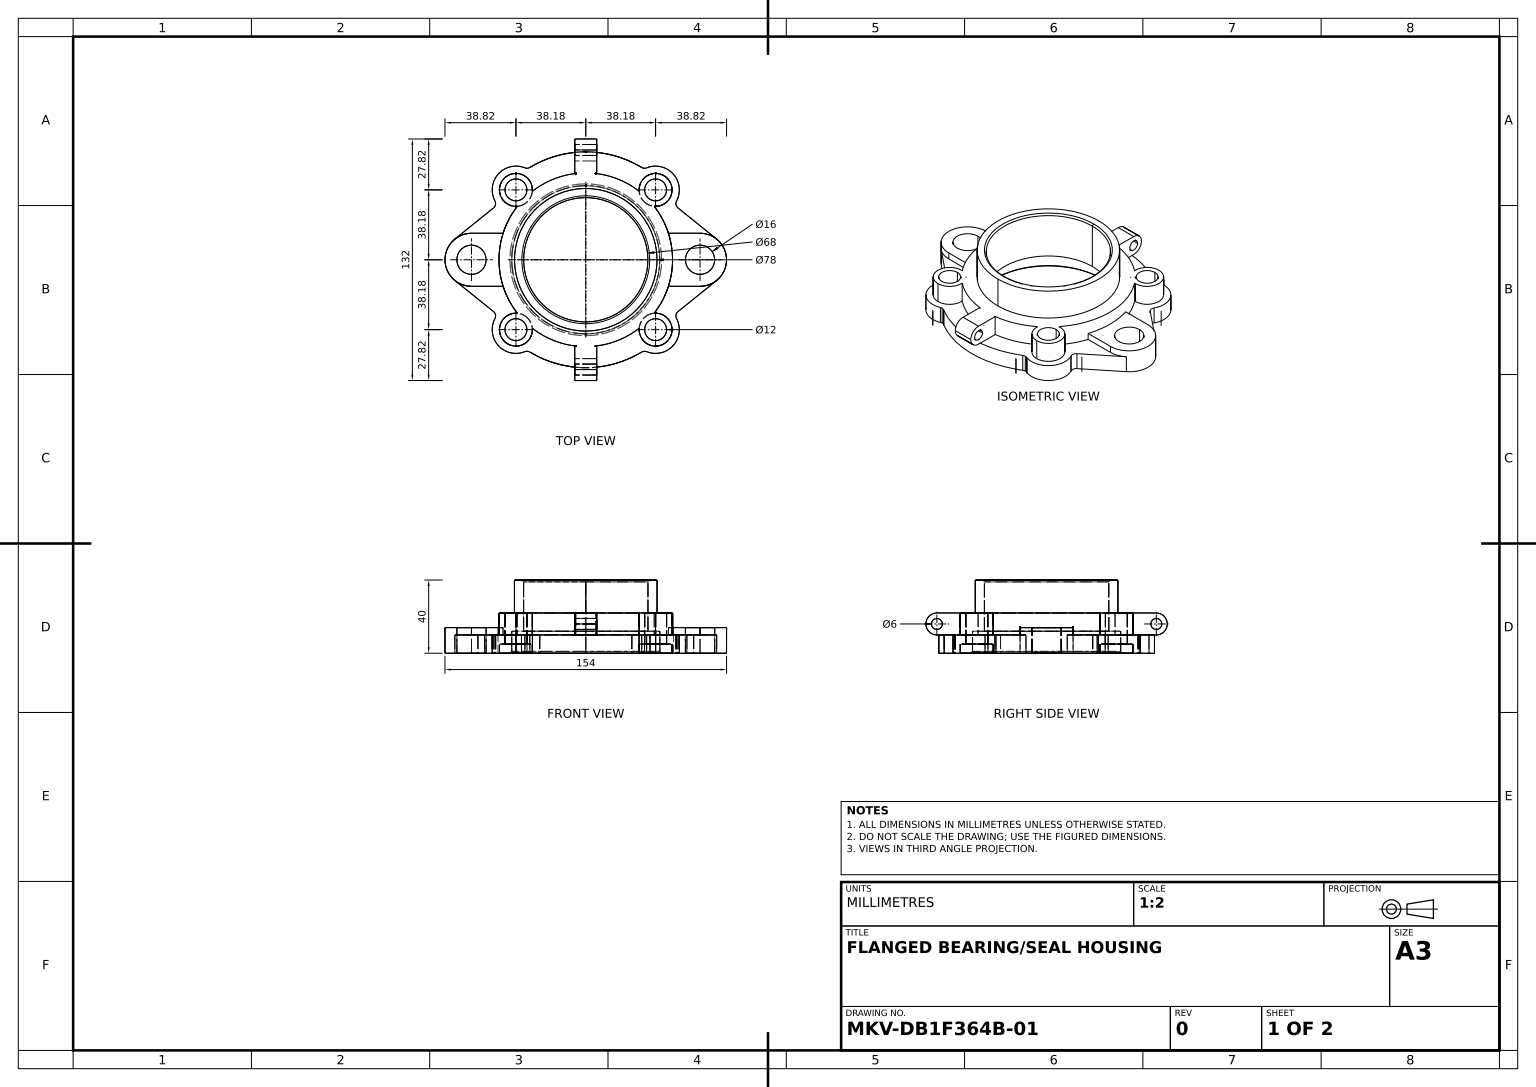
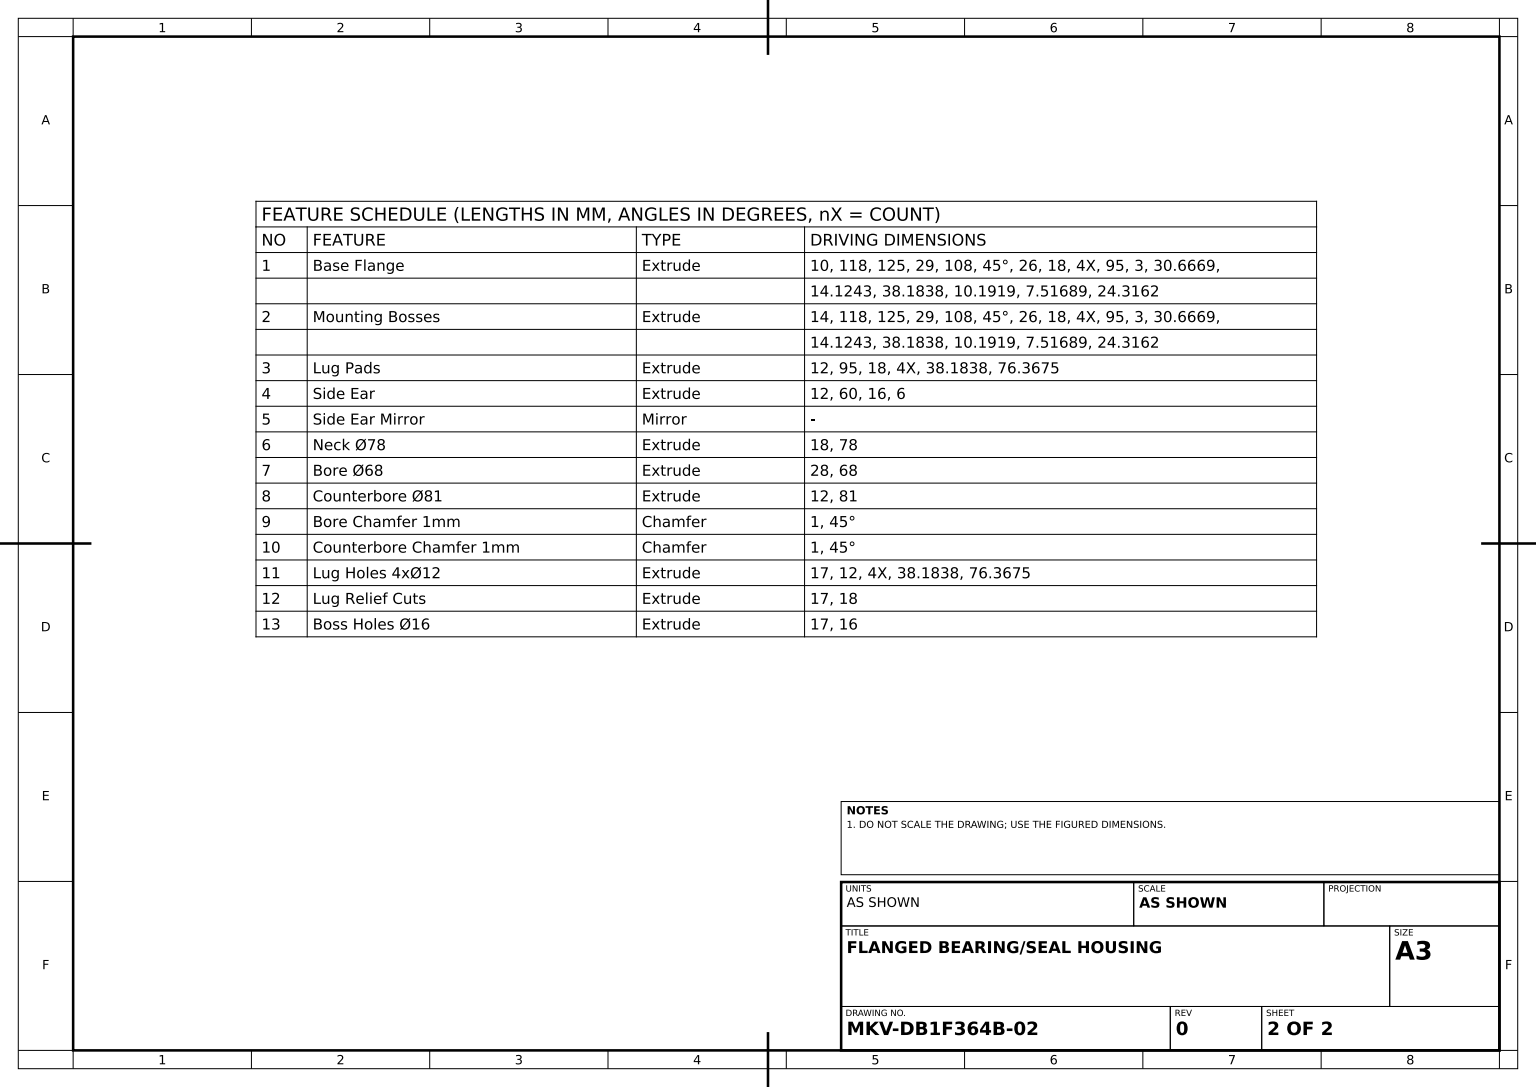
from build123d import *

# Parameters (mm, degrees)
BASE_FLANGE_DEPTH            = 10
MOUNTING_BOSSES_DEPTH        = 14
LUG_PADS_DEPTH               = 12
SIDE_EAR_SKETCH_R            = 3
SIDE_EAR_DEPTH               = 6
NECK_SKETCH_78_R             = 39
NECK_78_DEPTH                = 18
BORE_SKETCH_68_R             = 34
BORE_68_DEPTH                = 28
COUNTERBORE_SKETCH_81_R      = 40.5
COUNTERBORE_81_DEPTH         = 12
BORE_CHAMFER_1MM_SIZE        = 1
COUNTERBORE_CHAMFER_1MM_SIZE = 1
LUG_HOLES_SKETCH_R           = 6
LUG_HOLES_4X_12_DEPTH        = 17
LUG_START                    = -17
LUG_RELIEF_SKETCH_R          = 9
LUG_RELIEF_CUTS_DEPTH        = 17
BOSS_HOLES_SKETCH_R          = 8
BOSS_HOLES_16_DEPTH          = 17


with BuildPart() as part:
    # Base Flange Sketch → Base Flange (new body)
    with BuildSketch(Plane(origin=(0, 0, 0), x_dir=(1, 0, 0), z_dir=(0, 1, 0))):
        with BuildLine():
            Line((-45.232731512, -14.5), (-62.5, -14.5))
            ThreePointArc((-62.5, -14.5), (-67.319751251, -13.675525507), (-71.591397402, -11.295861777))
            Line((-71.591397402, -11.295861777), (-50.427104316, -28.329798892))
            ThreePointArc((-50.427104316, -28.329798892), (-49.36909282, -30.064930059), (-49.659773669, -32.076291075))
            ThreePointArc((-49.659773669, -32.076291075), (-47.837591407, -46.890295835), (-33.289777567, -50.227390033))
            ThreePointArc((-33.289777567, -50.227390033), (-31.921585171, -50.016208018), (-30.604247405, -50.44184811))
            ThreePointArc((-30.604247405, -50.44184811), (0, -59), (30.604247405, -50.44184811))
            ThreePointArc((30.604247405, -50.44184811), (31.921585171, -50.016208018), (33.289777567, -50.227390033))
            ThreePointArc((33.289777567, -50.227390033), (47.837591407, -46.890295835), (49.659773669, -32.076291075))
            ThreePointArc((49.659773669, -32.076291075), (49.36909282, -30.064930059), (50.427104316, -28.329798892))
            Line((50.427104316, -28.329798892), (71.591397402, -11.295861777))
            ThreePointArc((71.591397402, -11.295861777), (67.319751251, -13.675525507), (62.5, -14.5))
            Line((62.5, -14.5), (45.232731512, -14.5))
            ThreePointArc((45.232731512, -14.5), (43.022471721, -20.132484374), (40.114125183, -25.438297128))
            ThreePointArc((40.114125183, -25.438297128), (39.792711515, -27.966518872), (41.531678205, -29.829636361))
            ThreePointArc((41.531678205, -29.829636361), (44.547727215, -44.547727215), (29.829636361, -41.531678205))
            ThreePointArc((29.829636361, -41.531678205), (27.966518872, -39.792711515), (25.438297128, -40.114125183))
            ThreePointArc((25.438297128, -40.114125183), (0, -47.5), (-25.438297128, -40.114125183))
            ThreePointArc((-25.438297128, -40.114125183), (-27.966518872, -39.792711515), (-29.829636361, -41.531678205))
            ThreePointArc((-29.829636361, -41.531678205), (-44.547727215, -44.547727215), (-41.531678205, -29.829636361))
            ThreePointArc((-41.531678205, -29.829636361), (-39.792711515, -27.966518872), (-40.114125183, -25.438297128))
            ThreePointArc((-40.114125183, -25.438297128), (-43.022471721, -20.132484374), (-45.232731512, -14.5))
        make_face()
        with BuildLine():
            Line((-62.5, 14.5), (-45.232731512, 14.5))
            ThreePointArc((-45.232731512, 14.5), (-43.022471721, 20.132484374), (-40.114125183, 25.438297128))
            ThreePointArc((-40.114125183, 25.438297128), (-39.792711515, 27.966518872), (-41.531678205, 29.829636361))
            ThreePointArc((-41.531678205, 29.829636361), (-44.547727215, 44.547727215), (-29.829636361, 41.531678205))
            ThreePointArc((-29.829636361, 41.531678205), (-27.966518872, 39.792711515), (-25.438297128, 40.114125183))
            ThreePointArc((-25.438297128, 40.114125183), (0, 47.5), (25.438297128, 40.114125183))
            ThreePointArc((25.438297128, 40.114125183), (27.966518872, 39.792711515), (29.829636361, 41.531678205))
            ThreePointArc((29.829636361, 41.531678205), (44.547727215, 44.547727215), (41.531678205, 29.829636361))
            ThreePointArc((41.531678205, 29.829636361), (39.792711515, 27.966518872), (40.114125183, 25.438297128))
            ThreePointArc((40.114125183, 25.438297128), (43.022471721, 20.132484374), (45.232731512, 14.5))
            Line((45.232731512, 14.5), (62.5, 14.5))
            ThreePointArc((62.5, 14.5), (67.319751251, 13.675525507), (71.591397402, 11.295861777))
            Line((71.591397402, 11.295861777), (50.427104316, 28.329798892))
            ThreePointArc((50.427104316, 28.329798892), (49.36909282, 30.064930059), (49.659773669, 32.076291075))
            ThreePointArc((49.659773669, 32.076291075), (47.837591407, 46.890295835), (33.289777567, 50.227390033))
            ThreePointArc((33.289777567, 50.227390033), (31.921585171, 50.016208018), (30.604247405, 50.44184811))
            ThreePointArc((30.604247405, 50.44184811), (0, 59), (-30.604247405, 50.44184811))
            ThreePointArc((-30.604247405, 50.44184811), (-31.921585171, 50.016208018), (-33.289777567, 50.227390033))
            ThreePointArc((-33.289777567, 50.227390033), (-47.837591407, 46.890295835), (-49.659773669, 32.076291075))
            ThreePointArc((-49.659773669, 32.076291075), (-49.36909282, 30.064930059), (-50.427104316, 28.329798892))
            Line((-50.427104316, 28.329798892), (-71.591397402, 11.295861777))
            ThreePointArc((-71.591397402, 11.295861777), (-67.319751251, 13.675525507), (-62.5, 14.5))
        make_face()
        with BuildLine():
            ThreePointArc((-25.438297128, -40.114125183), (-27.966518872, -39.792711515), (-29.829636361, -41.531678205))
            ThreePointArc((-29.829636361, -41.531678205), (-44.547727215, -44.547727215), (-41.531678205, -29.829636361))
            ThreePointArc((-41.531678205, -29.829636361), (-39.792711515, -27.966518872), (-40.114125183, -25.438297128))
            ThreePointArc((-40.114125183, -25.438297128), (-47.5, 0), (-40.114125183, 25.438297128))
            ThreePointArc((-40.114125183, 25.438297128), (-39.792711515, 27.966518872), (-41.531678205, 29.829636361))
            ThreePointArc((-41.531678205, 29.829636361), (-44.547727215, 44.547727215), (-29.829636361, 41.531678205))
            ThreePointArc((-29.829636361, 41.531678205), (-27.966518872, 39.792711515), (-25.438297128, 40.114125183))
            ThreePointArc((-25.438297128, 40.114125183), (0, 47.5), (25.438297128, 40.114125183))
            ThreePointArc((25.438297128, 40.114125183), (27.966518872, 39.792711515), (29.829636361, 41.531678205))
            ThreePointArc((29.829636361, 41.531678205), (44.547727215, 44.547727215), (41.531678205, 29.829636361))
            ThreePointArc((41.531678205, 29.829636361), (39.792711515, 27.966518872), (40.114125183, 25.438297128))
            ThreePointArc((40.114125183, 25.438297128), (47.5, 0), (40.114125183, -25.438297128))
            ThreePointArc((40.114125183, -25.438297128), (39.792711515, -27.966518872), (41.531678205, -29.829636361))
            ThreePointArc((41.531678205, -29.829636361), (44.547727215, -44.547727215), (29.829636361, -41.531678205))
            ThreePointArc((29.829636361, -41.531678205), (27.966518872, -39.792711515), (25.438297128, -40.114125183))
            ThreePointArc((25.438297128, -40.114125183), (0, -47.5), (-25.438297128, -40.114125183))
        make_face()
    extrude(amount=BASE_FLANGE_DEPTH)

    # Sketch1_5 → Mounting Bosses (add)
    with BuildSketch(Plane(origin=(0, 0, 0), x_dir=(1, 0, 0), z_dir=(0, 1, 0))):
        with BuildLine():
            ThreePointArc((-71.591397402, -11.295861777), (-67.319751251, -13.675525507), (-62.5, -14.5))
            Line((-62.5, -14.5), (-45.232731512, -14.5))
            ThreePointArc((-45.232731512, -14.5), (-47.5, 0), (-45.232731512, 14.5))
            Line((-45.232731512, 14.5), (-62.5, 14.5))
            ThreePointArc((-62.5, 14.5), (-67.319751251, 13.675525507), (-71.591397402, 11.295861777))
            ThreePointArc((-71.591397402, 11.295861777), (-77, 0), (-71.591397402, -11.295861777))
        make_face()
        with BuildLine():
            ThreePointArc((45.232731512, 14.5), (47.5, 0), (45.232731512, -14.5))
            Line((45.232731512, -14.5), (62.5, -14.5))
            ThreePointArc((62.5, -14.5), (67.319751251, -13.675525507), (71.591397402, -11.295861777))
            ThreePointArc((71.591397402, -11.295861777), (77, 0), (71.591397402, 11.295861777))
            ThreePointArc((71.591397402, 11.295861777), (67.319751251, 13.675525507), (62.5, 14.5))
            Line((62.5, 14.5), (45.232731512, 14.5))
        make_face()
    extrude(amount=MOUNTING_BOSSES_DEPTH)

    # Lug Pads Sketch → Lug Pads (add)
    with BuildSketch(Plane(origin=(0, 10, 0), x_dir=(1, 0, 0), z_dir=(0, 1, 0))):
        with BuildLine():
            ThreePointArc((45.232731512, -14.5), (46.929759997, -7.338094208), (47.5, 0))
            ThreePointArc((47.5, 0), (46.929759997, 7.338094208), (45.232731512, 14.5))
            ThreePointArc((45.232731512, 14.5), (41.992969513, 22.200011521), (37.454357099, 29.213372526))
            ThreePointArc((37.454357099, 29.213372526), (33.587572106, 33.587572106), (29.213372526, 37.454357099))
            ThreePointArc((29.213372526, 37.454357099), (0, 47.5), (-29.213372526, 37.454357099))
            ThreePointArc((-29.213372526, 37.454357099), (-33.587572106, 33.587572106), (-37.454357099, 29.213372526))
            ThreePointArc((-37.454357099, 29.213372526), (-41.992969513, 22.200011521), (-45.232731512, 14.5))
            ThreePointArc((-45.232731512, 14.5), (-47.5, 0), (-45.232731512, -14.5))
            ThreePointArc((-45.232731512, -14.5), (-41.992969513, -22.200011521), (-37.454357099, -29.213372526))
            ThreePointArc((-37.454357099, -29.213372526), (-33.587572106, -33.587572106), (-29.213372526, -37.454357099))
            ThreePointArc((-29.213372526, -37.454357099), (0, -47.5), (29.213372526, -37.454357099))
            ThreePointArc((29.213372526, -37.454357099), (33.587572106, -33.587572106), (37.454357099, -29.213372526))
            ThreePointArc((37.454357099, -29.213372526), (41.992969513, -22.200011521), (45.232731512, -14.5))
        make_face()
        with BuildLine():
            ThreePointArc((-37.454357099, -29.213372526), (-44.547727215, -44.547727215), (-29.213372526, -37.454357099))
            ThreePointArc((-29.213372526, -37.454357099), (-33.587572106, -33.587572106), (-37.454357099, -29.213372526))
        make_face()
        with BuildLine():
            ThreePointArc((29.213372526, -37.454357099), (44.547727215, -44.547727215), (37.454357099, -29.213372526))
            ThreePointArc((37.454357099, -29.213372526), (33.587572106, -33.587572106), (29.213372526, -37.454357099))
        make_face()
        with BuildLine():
            ThreePointArc((29.213372526, 37.454357099), (33.587572106, 33.587572106), (37.454357099, 29.213372526))
            ThreePointArc((37.454357099, 29.213372526), (44.547727215, 44.547727215), (29.213372526, 37.454357099))
        make_face()
        with BuildLine():
            ThreePointArc((-37.454357099, 29.213372526), (-33.587572106, 33.587572106), (-29.213372526, 37.454357099))
            ThreePointArc((-29.213372526, 37.454357099), (-44.547727215, 44.547727215), (-37.454357099, 29.213372526))
        make_face()
    extrude(amount=LUG_PADS_DEPTH)

    # Side Ear Sketch → Side Ear (add, symmetric)
    with BuildSketch(Plane(origin=(0, 0, 0), x_dir=(0, 0, -1), z_dir=(1, 0, 0))):
        with BuildLine():
            Line((-60, 10), (-47.183766184, 10))
            Line((-47.183766184, 10), (-47.183766184, 22))
            Line((-47.183766184, 22), (-60, 22))
            ThreePointArc((-60, 22), (-66, 16), (-60, 10))
        make_face()
        with Locations((-60, 16)):
            Circle(SIDE_EAR_SKETCH_R, mode=Mode.SUBTRACT)
    side_ear = extrude(amount=SIDE_EAR_DEPTH, both=True)

    # Side Ear Mirror: Side Ear across plane
    add(side_ear.mirror(Plane.XY))

    # Neck Sketch _78 → Neck _78 (add)
    with BuildSketch(Plane(origin=(0, 22, 0), x_dir=(1, 0, 0), z_dir=(0, 1, 0))):
        with Locations(Location((0, 0, 0), (0, 0, 270))):
            Circle(NECK_SKETCH_78_R)
    extrude(amount=NECK_78_DEPTH)

    # Bore Sketch _68 → Bore _68 (cut)
    with BuildSketch(Plane(origin=(0, 40, 0), x_dir=(1, 0, 0), z_dir=(0, 1, 0))):
        with Locations(Location((0, 0, 0), (0, 0, 270))):
            Circle(BORE_SKETCH_68_R)
    extrude(amount=-BORE_68_DEPTH, mode=Mode.SUBTRACT)

    # Counterbore Sketch _81 → Counterbore _81 (cut)
    with BuildSketch(Plane(origin=(0, 12, 0), x_dir=(1, 0, 0), z_dir=(0, 1, 0))):
        with Locations(Location((0, 0, 0), (0, 0, 270))):
            Circle(COUNTERBORE_SKETCH_81_R)
    extrude(amount=-COUNTERBORE_81_DEPTH, mode=Mode.SUBTRACT)

    # Bore Chamfer 1mm
    bore_chamfer_1mm_edges = [part.edges().sort_by_distance(p)[0] for p in [
        (0, 40, -34),
    ]]
    chamfer(bore_chamfer_1mm_edges, length=BORE_CHAMFER_1MM_SIZE)

    # Counterbore Chamfer 1mm
    counterbore_chamfer_1mm_edges = [part.edges().sort_by_distance(p)[0] for p in [
        (0, 0, -40.5),
    ]]
    chamfer(counterbore_chamfer_1mm_edges, length=COUNTERBORE_CHAMFER_1MM_SIZE)

    # Lug Holes Sketch → Lug Holes 4x_12 (cut)
    with BuildSketch(Plane(origin=(0, 22, 0), x_dir=(1, 0, 0), z_dir=(0, 1, 0))):
        with Locations(Location((-38.183766184, 38.183766184, 0), (0, 0, 270))):
            Circle(LUG_HOLES_SKETCH_R)
        with Locations(Location((38.183766184, 38.183766184, 0), (0, 0, 270))):
            Circle(LUG_HOLES_SKETCH_R)
        with Locations(Location((38.183766184, -38.183766184, 0), (0, 0, 270))):
            Circle(LUG_HOLES_SKETCH_R)
        with Locations(Location((-38.183766184, -38.183766184, 0), (0, 0, 270))):
            Circle(LUG_HOLES_SKETCH_R)
    extrude(amount=-LUG_HOLES_4X_12_DEPTH, mode=Mode.SUBTRACT)

    # Lug Relief Sketch → Lug Relief Cuts (cut)
    with BuildSketch(Plane(origin=(0, 5, 0), x_dir=(1, 0, 0), z_dir=(0, 1, 0)).offset(LUG_START)):
        with Locations(Location((-38.183766184, 38.183766184, 0), (0, 0, 270))):
            Circle(LUG_RELIEF_SKETCH_R)
        with Locations(Location((38.183766184, 38.183766184, 0), (0, 0, 270))):
            Circle(LUG_RELIEF_SKETCH_R)
        with Locations(Location((38.183766184, -38.183766184, 0), (0, 0, 270))):
            Circle(LUG_RELIEF_SKETCH_R)
        with Locations(Location((-38.183766184, -38.183766184, 0), (0, 0, 270))):
            Circle(LUG_RELIEF_SKETCH_R)
    extrude(amount=LUG_RELIEF_CUTS_DEPTH, mode=Mode.SUBTRACT)

    # Boss Holes Sketch → Boss Holes _16 (cut)
    with BuildSketch(Plane(origin=(0, 14, 0), x_dir=(1, 0, 0), z_dir=(0, 1, 0))):
        with Locations(Location((-62.5, 0, 0), (0, 0, 270))):
            Circle(BOSS_HOLES_SKETCH_R)
        with Locations(Location((62.5, 0, 0), (0, 0, 270))):
            Circle(BOSS_HOLES_SKETCH_R)
    extrude(amount=-BOSS_HOLES_16_DEPTH, mode=Mode.SUBTRACT)


solid = part.part
